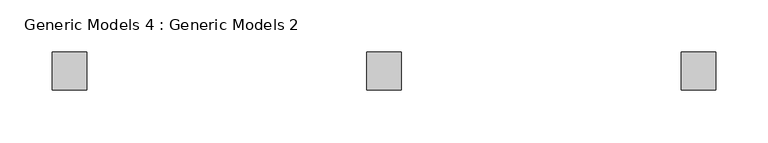
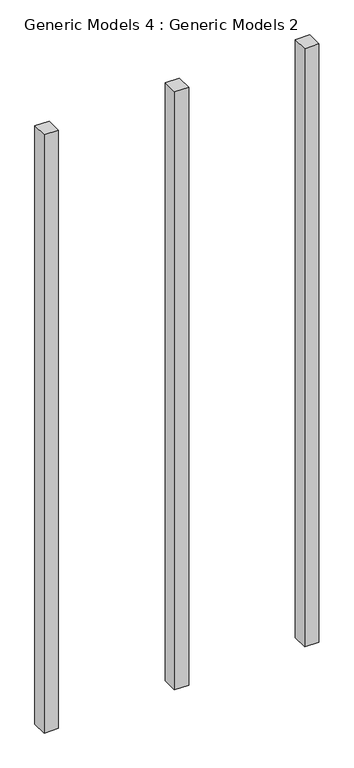
"""IFC4 building model written with IfcOpenShell, lengths in millimetres: proxy geometry, Generic Models 4 : Generic Models 2."""

from ifc_helpers import new_model, si_unit, frame, origin, place, context, project, spatial, polyline, outline, extrude, source, transform, mapped, element, save


def generic_models_4_generic_models_2_2859856a(model_context):
    return source(origin(), model_context, "Body", "SweptSolid", [
        extrude(outline(polyline([(-1624.0058248, -6197.2837816), (-1624.0058248, -6160.9896754), (-1591.1449896, -6160.9896754), (-1591.1449896, -6197.2837816), (-1624.0058248, -6197.2837816)])), frame((0.0, 0.0, -445.6320944), z_axis=(0.0, 0.0, 1.0), x_axis=(1.0, 0.0, 0.0)), (0.0, 0.0, 1.0), 1456.284726),
        extrude(outline(polyline([(-1924.0058248, -6197.2837816), (-1924.0058248, -6160.9896754), (-1891.1449896, -6160.9896754), (-1891.1449896, -6197.2837816), (-1924.0058248, -6197.2837816)])), frame((0.0, 0.0, -445.6320944), z_axis=(0.0, 0.0, 1.0), x_axis=(1.0, 0.0, 0.0)), (0.0, 0.0, 1.0), 1456.284726),
        extrude(outline(polyline([(-2224.0058248, -6197.2837816), (-2224.0058248, -6160.9896754), (-2191.1449896, -6160.9896754), (-2191.1449896, -6197.2837816), (-2224.0058248, -6197.2837816)])), frame((0.0, 0.0, -445.6320944), z_axis=(0.0, 0.0, 1.0), x_axis=(1.0, 0.0, 0.0)), (0.0, 0.0, 1.0), 1456.284726),
    ])


if __name__ == "__main__":
    model = new_model("IFC4")
    model_context = context("Model", 3, world=origin())
    ifc_project = project(units=[si_unit("LENGTHUNIT", "METRE", prefix="MILLI")], contexts=[model_context])
    site = spatial("IfcSite", under=ifc_project)
    building = spatial("IfcBuilding", under=site)
    placement = place(None, origin())
    generic_models_4_generic_models_2_shape = generic_models_4_generic_models_2_2859856a(model_context)
    element("IfcBuildingElementProxy", 1, Name="Generic Models 4 : Generic Models 2", ObjectType="Generic Models 4 : Generic Models 2", at=placement, inside=building, context=model_context, shape_type="MappedRepresentation", body=[
        mapped(generic_models_4_generic_models_2_shape, transform((0.0, 0.0, 0.0), x_axis=(1.0, 0.0, 0.0), y_axis=(0.0, 1.0, 0.0), z_axis=(0.0, 0.0, 1.0))),
    ])
    save(model, "model.ifc")
